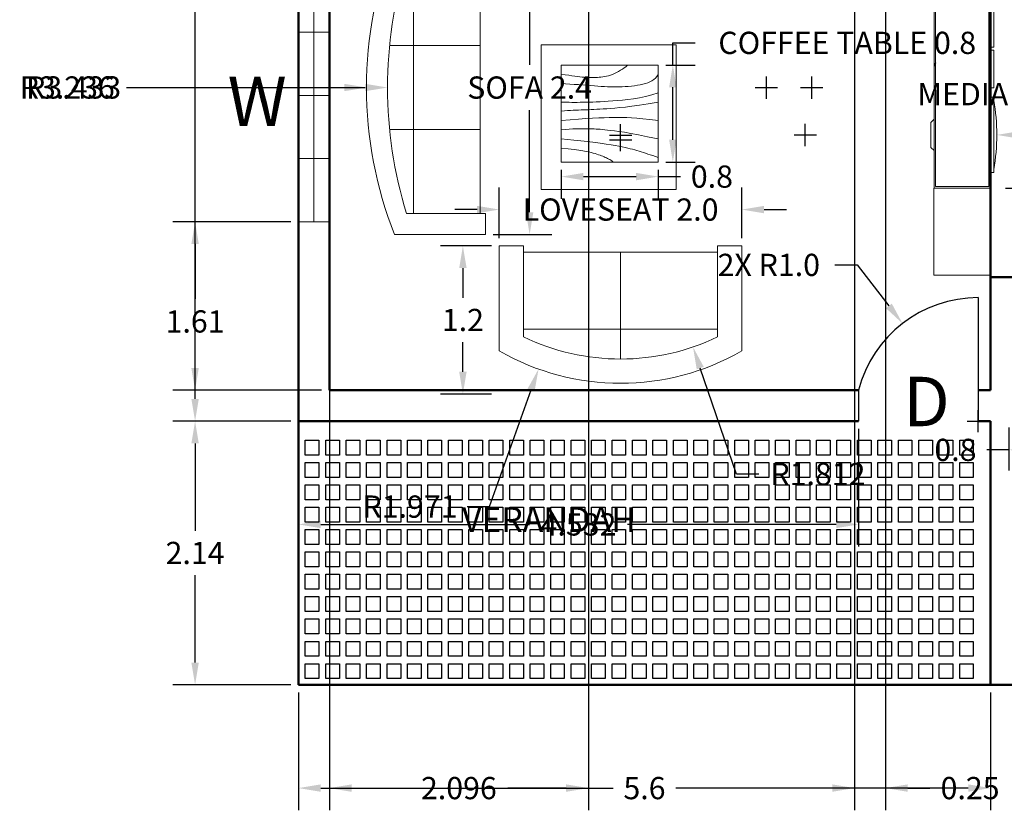
# Model space of a CAD drawing. Units: metres. Extents: x 3.9 to 21.3, y 24.8 to 56.5.
# Tile 1 of 6: x 3.9 to 11.9, y 24.8 to 31.2. Entities that reach past the tile are written whole.
import ezdxf

# ---------------------------------------------------------------- set-up
doc = ezdxf.new("R2010")
doc.units = ezdxf.units.M
doc.header["$MEASUREMENT"] = 0
for name, color, linetype, lineweight in [('A-AREA-IDEN', 3, 'Continuous', 25), ('A-FLOR-PATT', 8, 'Continuous', 13), ('DIMENSIONS', 2, 'Continuous', 18), ('DOOR', 5, 'Continuous', 25), ('FURNITURE', 6, 'Continuous', 18), ('TEXT', 3, 'Continuous', 18), ('WALL', 1, 'Continuous', 50), ('WINDOW', 4, 'Continuous', 18)]:
    doc.layers.add(name, color=color, linetype=linetype, lineweight=lineweight)
doc.styles.get("Standard").update_dxf_attribs({"font": 'arial.ttf'})
doc.dimstyles.get("Standard").update_dxf_attribs({"dimtxt": 0.18, "dimasz": 0.18, "dimexe": 0.18, "dimexo": 0.0625, "dimgap": 0.09, "dimtad": 0, "dimtih": 1, "dimtoh": 1, "dimdec": 1, "dimzin": 0, "dimdsep": 46, "dimtxsty": 'Standard', "dimcen": 0.09, "dimadec": 0, "dimazin": 0, "dimtfac": 1, "dimtdec": 1, "dimtofl": 0, "dimtmove": 0, "dimatfit": 3, "dimfxl": 1, "dimtolj": 1, "dimtzin": 0, "dimarcsym": 0})

# ---------------------------------------------------------------- blocks, each defined once
blk = doc.blocks.new('Entertainment Center')
for p, q in [((-4, 0), (-5, -1)), ((4, 0), (-4, 0)), ((5, -1), (4, 0)), ((-17, -19), (-17, -1)), ((-17, -1), (43, -1)), ((-16.5, -18.5), (-16.5, -1.5)), ((-16.5, -1.5), (42.5, -1.5)), ((42.5, -1.5), (42.5, -18.5)), ((43, -1), (43, -19)), ((42.5, -18.5), (-16.5, -18.5)), ((43, -19), (-17, -19)), ((-12, -20), (-12, -19)), ((12, -20), (-12, -20)), ((12, -19), (12, -20)), ((15, -20), (15, -19)), ((27, -20), (15, -20)), ((27, -19), (27, -20)), ((28, -20), (28, -19)), ((40, -20), (28, -20)), ((40, -19), (40, -20))]:
    blk.add_line(p, q)
blk.add_arc((0, 40), 61, 259.6111, 280.3889)
blk = doc.blocks.new('Sofa - Roundback 7 ft.')
for p, q in [((-12.00002, -32.4421), (-12.00003, -6.5971)), ((11.99997, -32.4421), (11.99998, -6.5971)), ((-36.000027, -34), (-36.000027, -11.4696)), ((-35.999844, -13.3819), (35.9998, -13.3819)), ((35.99998, -34), (35.99998, -11.4696)), ((-36.000027, -32.4421), (35.99998, -32.4421))]:
    blk.add_line(p, q)
for points in [[(-36.000027, -34), (-42.000027, -34), (-42.000027, -8)], [(41.99998, -8), (41.99998, -34), (35.99998, -34)]]:
    blk.add_lwpolyline(points)
for centre, radius, start, end in [((0, -114.25), 114.25, 68.43141, 111.5686), ((-0.00001, -127.1968), 121.1968, 72.72033, 107.2797)]:
    blk.add_arc(centre, radius, start, end)
blk = doc.blocks.new('Sofa - Roundback Loveseat 5 ft.')
for p, q in [((0, -32.44198), (0, -5.99998)), ((-24, -33.99998), (-24, -11.46958)), ((24.00004, -33.99998), (24.00004, -11.46958)), ((-23.9998, -13.38178), (23.99986, -13.38178)), ((-24, -32.44198), (24.00004, -32.44198))]:
    blk.add_line(p, q)
for points in [[(-24, -33.99998), (-30, -33.99998), (-30, -7.99998)], [(30.00004, -7.99998), (30.00004, -33.99998), (24.00004, -33.99998)]]:
    blk.add_lwpolyline(points)
for centre, radius, start, end in [((0, -60.24998), 60.24998, 60.13715, 119.8628), ((0, -61.38438), 55.38444, 64.32083, 115.6792)]:
    blk.add_arc(centre, radius, start, end)
blk = doc.blocks.new('Table - Square Woodgrain 42 x 42 in.')
blk.add_line((0, -42), (42, -42))
for points in [[(0, -4), (1.704, -4.2172), (3.2358, -4.4188), (4.615, -4.604), (5.8615, -4.7721), (6.9951, -4.9224), (8.0357, -5.0541), (9.0031, -5.1667), (9.9171, -5.2594), (10.7951, -5.3316), (11.6445, -5.3836), (12.4702, -5.4157), (13.277, -5.4283), (14.0698, -5.4217), (14.8535, -5.3964), (15.6331, -5.3526), (16.4133, -5.2908), (17.1986, -5.2103), (17.9913, -5.1062), (18.793, -4.9727), (19.6056, -4.8038), (20.4307, -4.5937), (21.2701, -4.3365), (22.1256, -4.0262), (22.9989, -3.6571), (23.888, -3.2272), (24.7756, -2.7516), (25.6408, -2.2491), (26.4624, -1.7387), (27.2195, -1.2395), (27.891, -0.7703), (28.456, -0.3501), (28.8934, 0.002)], [(0, -42), (0, 0), (42, 0), (42, -42)], [(0, -8), (1.8203, -8.1001), (3.6741, -8.2149), (5.5411, -8.3408), (7.4011, -8.4741), (9.2339, -8.6112), (11.0193, -8.7484), (12.7371, -8.8821), (14.3671, -9.0086), (15.8954, -9.1246), (17.3337, -9.2278), (18.6997, -9.3159), (20.0116, -9.387), (21.2871, -9.4389), (22.5442, -9.4696), (23.8008, -9.477), (25.0749, -9.459), (26.3791, -9.4137), (27.7049, -9.3403), (29.0383, -9.2382), (30.3655, -9.1068), (31.6728, -8.9455), (32.9461, -8.7535), (34.1717, -8.5304), (35.3358, -8.2756), (36.4268, -7.9863), (37.443, -7.6521), (38.3849, -7.2603), (39.253, -6.7986), (40.048, -6.2542), (40.7705, -5.6147), (41.421, -4.8674), (42, -4)], [(42, -12), (39.1784, -12.8621), (36.4519, -13.5654), (33.8246, -14.1294), (31.3004, -14.5731), (28.8832, -14.9161), (26.577, -15.1775), (24.3858, -15.3768), (22.3136, -15.5332), (20.3622, -15.6632), (18.5254, -15.7718), (16.7947, -15.8612), (15.1618, -15.9338), (13.6183, -15.9916), (12.1558, -16.0369), (10.7659, -16.0718), (9.4403, -16.0987), (8.1703, -16.1191), (6.9461, -16.1325), (5.7577, -16.1377), (4.595, -16.1335), (3.4479, -16.1188), (2.3064, -16.0924), (1.1604, -16.0532), (0, -16)], [(42, -16), (37.6529, -16.7365), (33.8802, -17.329), (30.6179, -17.7961), (27.8015, -18.1561), (25.3668, -18.4275), (23.2497, -18.6288), (21.3859, -18.7785), (19.7111, -18.8949), (18.1693, -18.9939), (16.7375, -19.0795), (15.401, -19.1534), (14.1449, -19.217), (12.9544, -19.2717), (11.8148, -19.3191), (10.7113, -19.3606), (9.6291, -19.3976), (8.5534, -19.4323), (7.47, -19.4689), (6.3643, -19.5122), (5.222, -19.5672), (4.0288, -19.6386), (2.7703, -19.7313), (1.4321, -19.8501), (0, -20)], [(0, -24), (3.9243, -23.6805), (7.4766, -23.4138), (10.6891, -23.1954), (13.5943, -23.0205), (16.2247, -22.8847), (18.6125, -22.7832), (20.7903, -22.7116), (22.7903, -22.6651), (24.6563, -22.642), (26.4764, -22.6507), (28.35, -22.7024), (30.3766, -22.8084), (32.6555, -22.98), (35.2861, -23.2283), (38.3678, -23.5645), (42, -24)], [(42, -32), (37.392, -31.017), (33.4585, -30.2231), (30.1291, -29.5949), (27.3334, -29.109), (25.0009, -28.742), (23.0612, -28.4707), (21.4439, -28.2716), (20.0786, -28.1215), (18.8998, -28.0002), (17.8609, -27.9014), (16.9206, -27.8219), (16.0371, -27.7588), (15.1691, -27.709), (14.2748, -27.6693), (13.3128, -27.6368), (12.2415, -27.6083), (11.0295, -27.5824), (9.6867, -27.5643), (8.233, -27.5608), (6.6884, -27.5787), (5.0728, -27.6248), (3.4062, -27.7058), (1.7086, -27.8286), (0, -28)], [(0, -32), (5.4026, -32.5358), (9.9494, -33.019), (13.7424, -33.4553), (16.8834, -33.8505), (19.4743, -34.2106), (21.6171, -34.5413), (23.4136, -34.8486), (24.9657, -35.1382), (26.3614, -35.4156), (27.6332, -35.6841), (28.7995, -35.9467), (29.8788, -36.2064), (30.8897, -36.4661), (31.8507, -36.7288), (32.7802, -36.9973), (33.6968, -37.2747), (34.6175, -37.5635), (35.5531, -37.8651), (36.5128, -38.1805), (37.506, -38.5108), (38.5421, -38.8568), (39.6302, -39.2197), (40.7797, -39.6004), (42, -40)], [(0, -36), (3.0098, -36.2857), (5.5354, -36.5643), (7.6368, -36.8359), (9.374, -37.1009), (10.807, -37.3597), (11.9957, -37.6126), (13.0002, -37.8599), (13.8804, -38.102), (14.6874, -38.3393), (15.4365, -38.5729), (16.1338, -38.8041), (16.7858, -39.0341), (17.3987, -39.264), (17.9787, -39.4952), (18.5322, -39.7288), (19.0655, -39.9662), (19.5832, -40.2081), (20.0842, -40.4544), (20.5657, -40.7046), (21.0249, -40.9581), (21.459, -41.2144), (21.8653, -41.4731), (22.2409, -41.7335), (22.5831, -41.9951)]]:
    blk.add_lwpolyline(points)
blk = doc.blocks.new('*U19')
at = {"layer": 'DOOR'}
blk.add_lwpolyline([(-0.0552, 0.0603), (0.0552, 0.0603), (0.0552, -0.0603), (-0.0552, -0.0603)], close=True, dxfattribs=at)
blk = doc.blocks.new('*U20')
at = {"layer": 'A-FLOR-PATT', "transparency": 16777216}
for p in [(0, 1.8102), (0.1655, 1.8102), (0.331, 1.8102), (0.4964, 1.8102), (0.6619, 1.8102), (0.8274, 1.8102), (0.9929, 1.8102), (1.1584, 1.8102), (1.3239, 1.8102), (1.4893, 1.8102), (1.6548, 1.8102), (1.8203, 1.8102), (1.9858, 1.8102), (2.1513, 1.8102), (2.3167, 1.8102), (2.4822, 1.8102), (2.6477, 1.8102), (2.8132, 1.8102), (2.9787, 1.8102), (3.1441, 1.8102), (3.3096, 1.8102), (3.4751, 1.8102), (3.6406, 1.8102), (3.8061, 1.8102), (3.9716, 1.8102), (4.137, 1.8102), (4.3025, 1.8102), (4.468, 1.8102), (4.6335, 1.8102), (4.799, 1.8102), (4.9644, 1.8102), (5.1299, 1.8102), (5.2954, 1.8102), (0, 1.6291), (0.1655, 1.6291), (0.331, 1.6291), (0.4964, 1.6291), (0.6619, 1.6291), (0.8274, 1.6291), (0.9929, 1.6291), (1.1584, 1.6291), (1.3239, 1.6291), (1.4893, 1.6291), (1.6548, 1.6291), (1.8203, 1.6291), (1.9858, 1.6291), (2.1513, 1.6291), (2.3167, 1.6291), (2.4822, 1.6291), (2.6477, 1.6291), (2.8132, 1.6291), (2.9787, 1.6291), (3.1441, 1.6291), (3.3096, 1.6291), (3.4751, 1.6291), (3.6406, 1.6291), (3.8061, 1.6291), (3.9716, 1.6291), (4.137, 1.6291), (4.3025, 1.6291), (4.468, 1.6291), (4.6335, 1.6291), (4.799, 1.6291), (4.9644, 1.6291), (5.1299, 1.6291), (5.2954, 1.6291), (0, 1.4481), (0.1655, 1.4481), (0.331, 1.4481), (0.4964, 1.4481), (0.6619, 1.4481), (0.8274, 1.4481), (0.9929, 1.4481), (1.1584, 1.4481), (1.3239, 1.4481), (1.4893, 1.4481), (1.6548, 1.4481), (1.8203, 1.4481), (1.9858, 1.4481), (2.1513, 1.4481), (2.3167, 1.4481), (2.4822, 1.4481), (2.6477, 1.4481), (2.8132, 1.4481), (2.9787, 1.4481), (3.1441, 1.4481), (3.3096, 1.4481), (3.4751, 1.4481), (3.6406, 1.4481), (3.8061, 1.4481), (3.9716, 1.4481), (4.137, 1.4481), (4.3025, 1.4481), (4.468, 1.4481), (4.6335, 1.4481), (4.799, 1.4481), (4.9644, 1.4481), (5.1299, 1.4481), (5.2954, 1.4481), (0, 1.2671), (0.1655, 1.2671), (0.331, 1.2671), (0.4964, 1.2671), (0.6619, 1.2671), (0.8274, 1.2671), (0.9929, 1.2671), (1.1584, 1.2671), (1.3239, 1.2671), (1.4893, 1.2671), (1.6548, 1.2671), (1.8203, 1.2671), (1.9858, 1.2671), (2.1513, 1.2671), (2.3167, 1.2671), (2.4822, 1.2671), (2.6477, 1.2671), (2.8132, 1.2671), (2.9787, 1.2671), (3.1441, 1.2671), (3.3096, 1.2671), (3.4751, 1.2671), (3.6406, 1.2671), (3.8061, 1.2671), (3.9716, 1.2671), (4.137, 1.2671), (4.3025, 1.2671), (4.468, 1.2671), (4.6335, 1.2671), (4.799, 1.2671), (4.9644, 1.2671), (5.1299, 1.2671), (5.2954, 1.2671), (0, 1.0861), (0.1655, 1.0861), (0.331, 1.0861), (0.4964, 1.0861), (0.6619, 1.0861), (0.8274, 1.0861), (0.9929, 1.0861), (1.1584, 1.0861), (1.3239, 1.0861), (1.4893, 1.0861), (1.6548, 1.0861), (1.8203, 1.0861), (1.9858, 1.0861), (2.1513, 1.0861), (2.3167, 1.0861), (2.4822, 1.0861), (2.6477, 1.0861), (2.8132, 1.0861), (2.9787, 1.0861), (3.1441, 1.0861), (3.3096, 1.0861), (3.4751, 1.0861), (3.6406, 1.0861), (3.8061, 1.0861), (3.9716, 1.0861), (4.137, 1.0861), (4.3025, 1.0861), (4.468, 1.0861), (4.6335, 1.0861), (4.799, 1.0861), (4.9644, 1.0861), (5.1299, 1.0861), (5.2954, 1.0861), (0, 0.9051), (0.1655, 0.9051), (0.331, 0.9051), (0.4964, 0.9051), (0.6619, 0.9051), (0.8274, 0.9051), (0.9929, 0.9051), (1.1584, 0.9051), (1.3239, 0.9051), (1.4893, 0.9051), (1.6548, 0.9051), (1.8203, 0.9051), (1.9858, 0.9051), (2.1513, 0.9051), (2.3167, 0.9051), (2.4822, 0.9051), (2.6477, 0.9051), (2.8132, 0.9051), (2.9787, 0.9051), (3.1441, 0.9051), (3.3096, 0.9051), (3.4751, 0.9051), (3.6406, 0.9051), (3.8061, 0.9051), (3.9716, 0.9051), (4.137, 0.9051), (4.3025, 0.9051), (4.468, 0.9051), (4.6335, 0.9051), (4.799, 0.9051), (4.9644, 0.9051), (5.1299, 0.9051), (5.2954, 0.9051), (0, 0.7241), (0.1655, 0.7241), (0.331, 0.7241), (0.4964, 0.7241), (0.6619, 0.7241), (0.8274, 0.7241), (0.9929, 0.7241), (1.1584, 0.7241), (1.3239, 0.7241), (1.4893, 0.7241), (1.6548, 0.7241), (1.8203, 0.7241), (1.9858, 0.7241), (2.1513, 0.7241), (2.3167, 0.7241), (2.4822, 0.7241), (2.6477, 0.7241), (2.8132, 0.7241), (2.9787, 0.7241), (3.1441, 0.7241), (3.3096, 0.7241), (3.4751, 0.7241), (3.6406, 0.7241), (3.8061, 0.7241), (3.9716, 0.7241), (4.137, 0.7241), (4.3025, 0.7241), (4.468, 0.7241), (4.6335, 0.7241), (4.799, 0.7241), (4.9644, 0.7241), (5.1299, 0.7241), (5.2954, 0.7241), (0, 0.543), (0.1655, 0.543), (0.331, 0.543), (0.4964, 0.543), (0.6619, 0.543), (0.8274, 0.543), (0.9929, 0.543), (1.1584, 0.543), (1.3239, 0.543), (1.4893, 0.543), (1.6548, 0.543), (1.8203, 0.543), (1.9858, 0.543), (2.1513, 0.543), (2.3167, 0.543), (2.4822, 0.543), (2.6477, 0.543), (2.8132, 0.543), (2.9787, 0.543), (3.1441, 0.543), (3.3096, 0.543), (3.4751, 0.543), (3.6406, 0.543), (3.8061, 0.543), (3.9716, 0.543), (4.137, 0.543), (4.3025, 0.543), (4.468, 0.543), (4.6335, 0.543), (4.799, 0.543), (4.9644, 0.543), (5.1299, 0.543), (5.2954, 0.543), (0, 0.362), (0.1655, 0.362), (0.331, 0.362), (0.4964, 0.362), (0.6619, 0.362), (0.8274, 0.362), (0.9929, 0.362), (1.1584, 0.362), (1.3239, 0.362), (1.4893, 0.362), (1.6548, 0.362), (1.8203, 0.362), (1.9858, 0.362), (2.1513, 0.362), (2.3167, 0.362), (2.4822, 0.362), (2.6477, 0.362), (2.8132, 0.362), (2.9787, 0.362), (3.1441, 0.362), (3.3096, 0.362), (3.4751, 0.362), (3.6406, 0.362), (3.8061, 0.362), (3.9716, 0.362), (4.137, 0.362), (4.3025, 0.362), (4.468, 0.362), (4.6335, 0.362), (4.799, 0.362), (4.9644, 0.362), (5.1299, 0.362), (5.2954, 0.362), (0, 0.181), (0.1655, 0.181), (0.331, 0.181), (0.4964, 0.181), (0.6619, 0.181), (0.8274, 0.181), (0.9929, 0.181), (1.1584, 0.181), (1.3239, 0.181), (1.4893, 0.181), (1.6548, 0.181), (1.8203, 0.181), (1.9858, 0.181), (2.1513, 0.181), (2.3167, 0.181), (2.4822, 0.181), (2.6477, 0.181), (2.8132, 0.181), (2.9787, 0.181), (3.1441, 0.181), (3.3096, 0.181), (3.4751, 0.181), (3.6406, 0.181), (3.8061, 0.181), (3.9716, 0.181), (4.137, 0.181), (4.3025, 0.181), (4.468, 0.181), (4.6335, 0.181), (4.799, 0.181), (4.9644, 0.181), (5.1299, 0.181), (5.2954, 0.181), (0, 0), (0.1655, 0), (0.331, 0), (0.4964, 0), (0.6619, 0), (0.8274, 0), (0.9929, 0), (1.1584, 0), (1.3239, 0), (1.4893, 0), (1.6548, 0), (1.8203, 0), (1.9858, 0), (2.1513, 0), (2.3167, 0), (2.4822, 0), (2.6477, 0), (2.8132, 0), (2.9787, 0), (3.1441, 0), (3.3096, 0), (3.4751, 0), (3.6406, 0), (3.8061, 0), (3.9716, 0), (4.137, 0), (4.3025, 0), (4.468, 0), (4.6335, 0), (4.799, 0), (4.9644, 0), (5.1299, 0), (5.2954, 0)]:
    blk.add_blockref('*U19', p, dxfattribs=at)
blk = doc.blocks.new('WIN-4-LIGHT-2046')
for p, q in [((0.5115, -0.125), (0, -0.125)), ((0.5115, -0.125), (1.0231, -0.125)), ((1.5346, -0.125), (1.0231, -0.125)), ((1.5346, -0.125), (2.0462, -0.125))]:
    blk.add_line(p, q)
for points in [[(0.5115, 0), (0, 0), (0, -0.25), (0.5115, -0.25)], [(0.5115, 0), (1.0231, 0), (1.0231, -0.25), (0.5115, -0.25)], [(1.5346, 0), (1.0231, 0), (1.0231, -0.25), (1.5346, -0.25)], [(1.5346, 0), (2.0462, 0), (2.0462, -0.25), (1.5346, -0.25)]]:
    blk.add_lwpolyline(points, close=True)
blk = doc.blocks.new('*D59')
at = {"layer": 'Defpoints', "color": 0, "transparency": 16777216}
for p in [(11.8164, 31.3903), (12.045, 31.3903), (11.8164, 29.8663)]:
    blk.add_point(p, dxfattribs=at)
at = {"layer": 'DIMENSIONS', "color": 0, "lineweight": -2, "transparency": 16777216}
for p, q in [((11.8789, 31.3903), (12.225, 31.3903)), ((12.045, 31.2103), (12.045, 30.8102)), ((12.045, 30.0463), (12.045, 30.4464)), ((11.8789, 29.8663), (12.225, 29.8663))]:
    blk.add_line(p, q, dxfattribs=at)
at = {"layer": 'DIMENSIONS', "color": 0, "transparency": 16777216}
for points in [[(12.015, 31.2103), (12.075, 31.2103), (12.045, 31.3903)], [(12.015, 30.0463), (12.075, 30.0463), (12.045, 29.8663)]]:
    blk.add_solid(points, dxfattribs=at)
at = {"layer": 'DIMENSIONS', "color": 0, "transparency": 16777216, "insert": (12.045, 30.6283), "char_height": 0.18, "attachment_point": 5}
blk.add_mtext('\\A1;MEDIA UNIT 1.5', dxfattribs=at)
blk = doc.blocks.new('*D61')
at = {"layer": 'Defpoints', "color": 0, "transparency": 16777216}
for p in [(7.6708, 31.8712), (8.0277, 31.8712), (7.6708, 29.4918)]:
    blk.add_point(p, dxfattribs=at)
at = {"layer": 'DIMENSIONS', "color": 0, "lineweight": -2, "transparency": 16777216}
for p, q in [((7.7333, 31.8712), (8.2077, 31.8712)), ((8.0277, 31.6912), (8.0277, 30.8646)), ((8.0277, 29.6718), (8.0277, 30.4984)), ((7.7333, 29.4918), (8.2077, 29.4918))]:
    blk.add_line(p, q, dxfattribs=at)
at = {"layer": 'DIMENSIONS', "color": 0, "transparency": 16777216}
for points in [[(7.9977, 31.6912), (8.0577, 31.6912), (8.0277, 31.8712)], [(7.9977, 29.6718), (8.0577, 29.6718), (8.0277, 29.4918)]]:
    blk.add_solid(points, dxfattribs=at)
at = {"layer": 'DIMENSIONS', "color": 0, "transparency": 16777216, "insert": (8.0277, 30.6815), "char_height": 0.18, "attachment_point": 5}
blk.add_mtext('\\A1;SOFA 2.4', dxfattribs=at)
blk = doc.blocks.new('*D63')
at = {"layer": 'Defpoints', "color": 0, "transparency": 16777216}
for p in [(7.7822, 29.6935), (7.7822, 29.399), (9.7451, 29.399)]:
    blk.add_point(p, dxfattribs=at)
at = {"layer": 'DIMENSIONS', "color": 0, "lineweight": -2, "transparency": 16777216}
for p, q in [((7.7822, 29.4615), (7.7822, 29.8735)), ((9.7451, 29.4615), (9.7451, 29.8735)), ((7.6022, 29.6935), (7.4222, 29.6935)), ((9.9251, 29.6935), (10.1051, 29.6935))]:
    blk.add_line(p, q, dxfattribs=at)
at = {"layer": 'DIMENSIONS', "color": 0, "transparency": 16777216}
for points in [[(7.6022, 29.7235), (7.6022, 29.6635), (7.7822, 29.6935)], [(9.9251, 29.7235), (9.9251, 29.6635), (9.7451, 29.6935)]]:
    blk.add_solid(points, dxfattribs=at)
at = {"layer": 'DIMENSIONS', "color": 0, "transparency": 16777216, "insert": (8.7636, 29.6935), "char_height": 0.18, "attachment_point": 5}
blk.add_mtext('\\A1;LOVESEAT 2.0', dxfattribs=at)
blk = doc.blocks.new('*D64')
at = {"layer": 'Defpoints', "color": 0, "transparency": 16777216}
for p in [(7.7822, 29.399), (7.4878, 28.1995), (7.7822, 28.1995)]:
    blk.add_point(p, dxfattribs=at)
at = {"layer": 'DIMENSIONS', "color": 0, "lineweight": -2, "transparency": 16777216}
for p, q in [((7.7197, 29.399), (7.3078, 29.399)), ((7.4878, 29.219), (7.4878, 28.9797)), ((7.4878, 28.3795), (7.4878, 28.6189)), ((7.7197, 28.1995), (7.3078, 28.1995))]:
    blk.add_line(p, q, dxfattribs=at)
at = {"layer": 'DIMENSIONS', "color": 0, "transparency": 16777216}
for points in [[(7.4578, 29.219), (7.5178, 29.219), (7.4878, 29.399)], [(7.4578, 28.3795), (7.5178, 28.3795), (7.4878, 28.1995)]]:
    blk.add_solid(points, dxfattribs=at)
at = {"layer": 'DIMENSIONS', "color": 0, "transparency": 16777216, "insert": (7.4878, 28.7993), "char_height": 0.18, "attachment_point": 5}
blk.add_mtext('\\A1;1.2', dxfattribs=at)
blk = doc.blocks.new('*D65')
at = {"layer": 'Defpoints', "color": 0, "transparency": 16777216}
for p in [(9.0686, 30.8635), (9.1864, 30.8635), (9.0686, 30.0783)]:
    blk.add_point(p, dxfattribs=at)
at = {"layer": 'DIMENSIONS', "color": 0, "lineweight": -2, "transparency": 16777216}
for p, q in [((9.1864, 30.8635), (9.1864, 31.0435)), ((9.1864, 31.0435), (9.3664, 31.0435)), ((9.1311, 30.8635), (9.3664, 30.8635)), ((9.1864, 30.2583), (9.1864, 30.6835)), ((9.1311, 30.0783), (9.3664, 30.0783))]:
    blk.add_line(p, q, dxfattribs=at)
at = {"layer": 'DIMENSIONS', "color": 0, "transparency": 16777216}
for points in [[(9.1564, 30.6835), (9.2164, 30.6835), (9.1864, 30.8635)], [(9.1564, 30.2583), (9.2164, 30.2583), (9.1864, 30.0783)]]:
    blk.add_solid(points, dxfattribs=at)
at = {"layer": 'DIMENSIONS', "color": 0, "transparency": 16777216, "insert": (10.5975, 31.0435), "char_height": 0.18, "attachment_point": 5}
blk.add_mtext('\\A1;COFFEE TABLE 0.8', dxfattribs=at)
blk = doc.blocks.new('*D66')
at = {"layer": 'Defpoints', "color": 0, "transparency": 16777216}
for p in [(8.2835, 30.0783), (9.0686, 30.0783), (9.0686, 29.9605)]:
    blk.add_point(p, dxfattribs=at)
at = {"layer": 'DIMENSIONS', "color": 0, "lineweight": -2, "transparency": 16777216}
for p, q in [((8.2835, 30.0158), (8.2835, 29.7805)), ((8.4635, 29.9605), (8.8886, 29.9605)), ((9.0686, 30.0158), (9.0686, 29.7805)), ((9.0686, 29.9605), (9.2486, 29.9605))]:
    blk.add_line(p, q, dxfattribs=at)
at = {"layer": 'DIMENSIONS', "color": 0, "transparency": 16777216}
for points in [[(8.4635, 29.9905), (8.4635, 29.9305), (8.2835, 29.9605)], [(8.8886, 29.9905), (8.8886, 29.9305), (9.0686, 29.9605)]]:
    blk.add_solid(points, dxfattribs=at)
at = {"layer": 'DIMENSIONS', "color": 0, "transparency": 16777216, "insert": (9.5027, 29.9605), "char_height": 0.18, "attachment_point": 5}
blk.add_mtext('\\A1;0.8', dxfattribs=at)
blk = doc.blocks.new('*D72')
at = {"layer": 'Defpoints', "color": 0, "transparency": 16777216}
for p in [(11.9074, 27.7476), (11.9074, 27.519), (12.6694, 27.519)]:
    blk.add_point(p, dxfattribs=at)
at = {"layer": 'DIMENSIONS', "color": 0, "lineweight": -2, "transparency": 16777216}
for p, q in [((11.9074, 27.5815), (11.9074, 27.9276)), ((12.6694, 27.5815), (12.6694, 27.9276)), ((11.9074, 27.7476), (11.7274, 27.7476)), ((12.4894, 27.7476), (12.0874, 27.7476))]:
    blk.add_line(p, q, dxfattribs=at)
at = {"layer": 'DIMENSIONS', "color": 0, "transparency": 16777216}
for points in [[(12.0874, 27.7776), (12.0874, 27.7176), (11.9074, 27.7476)], [(12.4894, 27.7776), (12.4894, 27.7176), (12.6694, 27.7476)]]:
    blk.add_solid(points, dxfattribs=at)
at = {"layer": 'DIMENSIONS', "color": 0, "transparency": 16777216, "insert": (11.4733, 27.7476), "char_height": 0.18, "attachment_point": 5}
blk.add_mtext('\\A1;0.8', dxfattribs=at)
blk = doc.blocks.new('*D73')
at = {"layer": 'Defpoints', "color": 0, "transparency": 16777216}
for p in [(5.3206, 27.9803), (6.1571, 27.9803), (6.1571, 25.8451)]:
    blk.add_point(p, dxfattribs=at)
at = {"layer": 'DIMENSIONS', "color": 0, "lineweight": -2, "transparency": 16777216}
for p, q in [((6.0946, 27.9803), (5.1406, 27.9803)), ((5.3206, 27.8003), (5.3206, 27.0931)), ((5.3206, 26.0251), (5.3206, 26.7323)), ((6.0946, 25.8451), (5.1406, 25.8451))]:
    blk.add_line(p, q, dxfattribs=at)
at = {"layer": 'DIMENSIONS', "color": 0, "transparency": 16777216}
for points in [[(5.2906, 27.8003), (5.3506, 27.8003), (5.3206, 27.9803)], [(5.2906, 26.0251), (5.3506, 26.0251), (5.3206, 25.8451)]]:
    blk.add_solid(points, dxfattribs=at)
at = {"layer": 'DIMENSIONS', "color": 0, "transparency": 16777216, "insert": (5.3206, 26.9127), "char_height": 0.18, "attachment_point": 5}
blk.add_mtext('\\A1;2.14', dxfattribs=at)
blk = doc.blocks.new('*D74')
at = {"layer": 'Defpoints', "color": 0, "transparency": 16777216}
for p in [(6.1571, 25.8451), (11.7571, 25.8451), (11.7571, 25.0086)]:
    blk.add_point(p, dxfattribs=at)
at = {"layer": 'DIMENSIONS', "color": 0, "lineweight": -2, "transparency": 16777216}
for p, q in [((6.1571, 25.7826), (6.1571, 24.8286)), ((11.7571, 25.7826), (11.7571, 24.8286)), ((6.3371, 25.0086), (8.7033, 25.0086)), ((11.5771, 25.0086), (9.2109, 25.0086))]:
    blk.add_line(p, q, dxfattribs=at)
at = {"layer": 'DIMENSIONS', "color": 0, "transparency": 16777216}
for points in [[(6.3371, 25.0386), (6.3371, 24.9786), (6.1571, 25.0086)], [(11.5771, 25.0386), (11.5771, 24.9786), (11.7571, 25.0086)]]:
    blk.add_solid(points, dxfattribs=at)
at = {"layer": 'DIMENSIONS', "color": 0, "transparency": 16777216, "insert": (8.9571, 25.0086), "char_height": 0.18, "attachment_point": 5}
blk.add_mtext('\\A1;5.6', dxfattribs=at)
blk = doc.blocks.new('*D76')
at = {"layer": 'Defpoints', "color": 0, "transparency": 16777216}
for p in [(6.4071, 38.6451), (5.3206, 28.2303), (6.4071, 28.2303)]:
    blk.add_point(p, dxfattribs=at)
at = {"layer": 'DIMENSIONS', "color": 0, "lineweight": -2, "transparency": 16777216}
for p, q in [((6.3446, 38.6451), (5.1406, 38.6451)), ((5.3206, 38.4651), (5.3206, 33.6196)), ((5.3206, 28.4103), (5.3206, 33.2558)), ((6.3446, 28.2303), (5.1406, 28.2303))]:
    blk.add_line(p, q, dxfattribs=at)
at = {"layer": 'DIMENSIONS', "color": 0, "transparency": 16777216}
for points in [[(5.2906, 38.4651), (5.3506, 38.4651), (5.3206, 38.6451)], [(5.2906, 28.4103), (5.3506, 28.4103), (5.3206, 28.2303)]]:
    blk.add_solid(points, dxfattribs=at)
at = {"layer": 'DIMENSIONS', "color": 0, "transparency": 16777216, "insert": (5.3206, 33.4377), "char_height": 0.18, "attachment_point": 5}
blk.add_mtext('\\A1;10.415', dxfattribs=at)
blk = doc.blocks.new('*D79')
at = {"layer": 'Defpoints', "color": 0, "transparency": 16777216}
for p in [(10.6571, 32.2457), (10.9071, 32.2457), (10.9071, 25.0086)]:
    blk.add_point(p, dxfattribs=at)
at = {"layer": 'DIMENSIONS', "color": 0, "lineweight": -2, "transparency": 16777216}
for p, q in [((10.6571, 32.1832), (10.6571, 24.8286)), ((10.9071, 32.1832), (10.9071, 24.8286)), ((10.4771, 25.0086), (10.2971, 25.0086)), ((11.0871, 25.0086), (11.2671, 25.0086))]:
    blk.add_line(p, q, dxfattribs=at)
at = {"layer": 'DIMENSIONS', "color": 0, "transparency": 16777216}
for points in [[(10.4771, 25.0386), (10.4771, 24.9786), (10.6571, 25.0086)], [(11.0871, 25.0386), (11.0871, 24.9786), (10.9071, 25.0086)]]:
    blk.add_solid(points, dxfattribs=at)
at = {"layer": 'DIMENSIONS', "color": 0, "transparency": 16777216, "insert": (11.5916, 25.0086), "char_height": 0.18, "attachment_point": 5}
blk.add_mtext('\\A1;0.25', dxfattribs=at)
blk = doc.blocks.new('*D91')
at = {"layer": 'Defpoints', "color": 0, "transparency": 16777216}
for p in [(5.3206, 29.5947), (6.1571, 29.5947), (6.1571, 27.9803)]:
    blk.add_point(p, dxfattribs=at)
at = {"layer": 'DIMENSIONS', "color": 0, "lineweight": -2, "transparency": 16777216}
for p, q in [((6.0946, 29.5947), (5.1406, 29.5947)), ((5.3206, 29.4147), (5.3206, 28.9694)), ((5.3206, 28.1603), (5.3206, 28.6056)), ((6.0946, 27.9803), (5.1406, 27.9803))]:
    blk.add_line(p, q, dxfattribs=at)
at = {"layer": 'DIMENSIONS', "color": 0, "transparency": 16777216}
for points in [[(5.2906, 29.4147), (5.3506, 29.4147), (5.3206, 29.5947)], [(5.2906, 28.1603), (5.3506, 28.1603), (5.3206, 27.9803)]]:
    blk.add_solid(points, dxfattribs=at)
at = {"layer": 'DIMENSIONS', "color": 0, "transparency": 16777216, "insert": (5.3206, 28.7875), "char_height": 0.18, "attachment_point": 5}
blk.add_mtext('\\A1;1.61', dxfattribs=at)
blk = doc.blocks.new('*D96')
at = {"layer": 'Defpoints', "color": 0, "transparency": 16777216}
for p in [(6.4071, 35.5686), (8.5033, 35.5686), (8.5033, 25.0086)]:
    blk.add_point(p, dxfattribs=at)
at = {"layer": 'DIMENSIONS', "color": 0, "lineweight": -2, "transparency": 16777216}
for p, q in [((6.4071, 35.5061), (6.4071, 24.8286)), ((8.5033, 35.5061), (8.5033, 24.8286)), ((6.5871, 25.0086), (7.06, 25.0086)), ((8.3233, 25.0086), (7.8504, 25.0086))]:
    blk.add_line(p, q, dxfattribs=at)
at = {"layer": 'DIMENSIONS', "color": 0, "transparency": 16777216}
for points in [[(6.5871, 25.0386), (6.5871, 24.9786), (6.4071, 25.0086)], [(8.3233, 25.0386), (8.3233, 24.9786), (8.5033, 25.0086)]]:
    blk.add_solid(points, dxfattribs=at)
at = {"layer": 'DIMENSIONS', "color": 0, "transparency": 16777216, "insert": (7.4552, 25.0086), "char_height": 0.18, "attachment_point": 5}
blk.add_mtext('\\A1;2.096', dxfattribs=at)
blk = doc.blocks.new('*D101')
at = {"layer": 'Defpoints', "color": 0, "transparency": 16777216}
for p in [(6.1571, 27.9803), (10.6889, 27.9803), (6.1571, 27.1438)]:
    blk.add_point(p, dxfattribs=at)
at = {"layer": 'DIMENSIONS', "color": 0, "lineweight": -2, "transparency": 16777216}
for p, q in [((6.1571, 27.9178), (6.1571, 26.9638)), ((10.6889, 27.9178), (10.6889, 26.9638)), ((6.3371, 27.1438), (8.0266, 27.1438)), ((10.5089, 27.1438), (8.8194, 27.1438))]:
    blk.add_line(p, q, dxfattribs=at)
at = {"layer": 'DIMENSIONS', "color": 0, "transparency": 16777216}
for points in [[(6.3371, 27.1738), (6.3371, 27.1138), (6.1571, 27.1438)], [(10.5089, 27.1738), (10.5089, 27.1138), (10.6889, 27.1438)]]:
    blk.add_solid(points, dxfattribs=at)
at = {"layer": 'DIMENSIONS', "color": 0, "transparency": 16777216, "insert": (8.423, 27.1438), "char_height": 0.18, "attachment_point": 5}
blk.add_mtext('\\A1;4.532', dxfattribs=at)
blk = doc.blocks.new('*D103')
at = {"layer": 'Defpoints', "color": 0, "transparency": 16777216}
for p in [(11.045, 28.771), (11.6571, 27.9803)]:
    blk.add_point(p, dxfattribs=at)
at = {"layer": 'DIMENSIONS', "color": 0, "lineweight": -2, "transparency": 16777216}
for p, q in [((10.4977, 29.2455), (10.6777, 29.2455)), ((10.6777, 29.2455), (10.9348, 28.9134)), ((11.6571, 27.8903), (11.6571, 28.0703)), ((11.5671, 27.9803), (11.7471, 27.9803))]:
    blk.add_line(p, q, dxfattribs=at)
at = {"layer": 'DIMENSIONS', "color": 0, "transparency": 16777216}
blk.add_solid([(10.9585, 28.9317), (10.9111, 28.895), (11.045, 28.771)], dxfattribs=at)
at = {"layer": 'DIMENSIONS', "color": 0, "transparency": 16777216, "insert": (9.9631, 29.2455), "char_height": 0.18, "attachment_point": 5}
blk.add_mtext('\\A1;2X R1.0', dxfattribs=at)
blk = doc.blocks.new('*D107')
at = {"layer": 'Defpoints', "color": 0, "transparency": 16777216}
for p in [(6.8776, 30.682), (10.3106, 30.6815)]:
    blk.add_point(p, dxfattribs=at)
at = {"layer": 'DIMENSIONS', "color": 0, "lineweight": -2, "transparency": 16777216}
for p, q in [((10.3106, 30.5915), (10.3106, 30.7715)), ((4.8178, 30.6823), (6.6976, 30.682)), ((10.2206, 30.6815), (10.4006, 30.6815))]:
    blk.add_line(p, q, dxfattribs=at)
at = {"layer": 'DIMENSIONS', "color": 0, "transparency": 16777216}
blk.add_solid([(6.6976, 30.712), (6.6976, 30.652), (6.8776, 30.682)], dxfattribs=at)
at = {"layer": 'DIMENSIONS', "color": 0, "transparency": 16777216, "insert": (4.338, 30.6823), "char_height": 0.18, "attachment_point": 5}
blk.add_mtext('\\A1;R3.433', dxfattribs=at)
blk = doc.blocks.new('*D108')
at = {"layer": 'Defpoints', "color": 0, "transparency": 16777216}
for p in [(6.7077, 30.682), (9.9439, 30.6815)]:
    blk.add_point(p, dxfattribs=at)
at = {"layer": 'DIMENSIONS', "color": 0, "lineweight": -2, "transparency": 16777216}
for p, q in [((9.9439, 30.5915), (9.9439, 30.7715)), ((4.7659, 30.6823), (6.5277, 30.682)), ((9.8539, 30.6815), (10.0339, 30.6815))]:
    blk.add_line(p, q, dxfattribs=at)
at = {"layer": 'DIMENSIONS', "color": 0, "transparency": 16777216}
blk.add_solid([(6.5277, 30.712), (6.5277, 30.652), (6.7077, 30.682)], dxfattribs=at)
at = {"layer": 'DIMENSIONS', "color": 0, "transparency": 16777216, "insert": (4.2862, 30.6823), "char_height": 0.18, "attachment_point": 5}
blk.add_mtext('\\A1;R3.236', dxfattribs=at)
blk = doc.blocks.new('*D109')
at = {"layer": 'Defpoints', "color": 0, "transparency": 16777216}
for p in [(8.7636, 30.2578), (8.1, 28.4019)]:
    blk.add_point(p, dxfattribs=at)
at = {"layer": 'DIMENSIONS', "color": 0, "lineweight": -2, "transparency": 16777216}
for p, q in [((8.7636, 30.1678), (8.7636, 30.3478)), ((8.6736, 30.2578), (8.8536, 30.2578)), ((7.7017, 27.2883), (8.0393, 28.2324)), ((7.5217, 27.2883), (7.7017, 27.2883))]:
    blk.add_line(p, q, dxfattribs=at)
at = {"layer": 'DIMENSIONS', "color": 0, "transparency": 16777216}
blk.add_solid([(8.0111, 28.2425), (8.0676, 28.2223), (8.1, 28.4019)], dxfattribs=at)
at = {"layer": 'DIMENSIONS', "color": 0, "transparency": 16777216, "insert": (7.0593, 27.2883), "char_height": 0.18, "attachment_point": 5}
blk.add_mtext('\\A1;R1.971', dxfattribs=at)
blk = doc.blocks.new('*D110')
at = {"layer": 'Defpoints', "color": 0, "transparency": 16777216}
for p in [(8.7636, 30.2949), (9.3498, 28.5805)]:
    blk.add_point(p, dxfattribs=at)
at = {"layer": 'DIMENSIONS', "color": 0, "lineweight": -2, "transparency": 16777216}
for p, q in [((8.7636, 30.2049), (8.7636, 30.3849)), ((8.6736, 30.2949), (8.8536, 30.2949)), ((9.7015, 27.5519), (9.4081, 28.4102)), ((9.8815, 27.5519), (9.7015, 27.5519))]:
    blk.add_line(p, q, dxfattribs=at)
at = {"layer": 'DIMENSIONS', "color": 0, "transparency": 16777216}
blk.add_solid([(9.4365, 28.4199), (9.3797, 28.4005), (9.3498, 28.5805)], dxfattribs=at)
at = {"layer": 'DIMENSIONS', "color": 0, "transparency": 16777216, "insert": (10.3605, 27.5519), "char_height": 0.18, "attachment_point": 5}
blk.add_mtext('\\A1;R1.812', dxfattribs=at)
blk = doc.blocks.new('*D111')
at = {"layer": 'Defpoints', "color": 0, "transparency": 16777216}
for p in [(10.2586, 30.2981), (11.808, 30.298)]:
    blk.add_point(p, dxfattribs=at)
at = {"layer": 'DIMENSIONS', "color": 0, "lineweight": -2, "transparency": 16777216}
for p, q in [((10.2586, 30.2081), (10.2586, 30.3881)), ((10.1686, 30.2981), (10.3486, 30.2981)), ((12.7376, 30.2979), (11.988, 30.298))]:
    blk.add_line(p, q, dxfattribs=at)
at = {"layer": 'DIMENSIONS', "color": 0, "transparency": 16777216}
blk.add_solid([(11.988, 30.328), (11.988, 30.268), (11.808, 30.298)], dxfattribs=at)
at = {"layer": 'DIMENSIONS', "color": 0, "transparency": 16777216, "insert": (13.1482, 30.2979), "char_height": 0.18, "attachment_point": 5}
blk.add_mtext('\\A1;R1.55', dxfattribs=at)

msp = doc.modelspace()

# ---------------------------------------------------------------- linework, layer by layer
at = {"layer": 'DOOR'}
for p, q in [((11.6571, 28.9803), (11.6571, 27.9803)), ((10.6889, 28.2303), (10.6889, 27.9803))]:
    msp.add_line(p, q, dxfattribs=at)
for centre, radius, start, end in [((12.1168, 30.4682), 0.904, 152.82202, 154.64088), ((11.6571, 27.9803), 1, 90, 165.52249)]:
    msp.add_arc(centre, radius, start, end, dxfattribs=at)
at = {"layer": 'FURNITURE'}
for points in [[(8.1215, 31.0287), (9.2141, 31.0287), (9.2141, 29.8547), (8.1215, 29.8547)], [(11.7572, 29.8663), (11.2972, 29.8663), (11.2972, 29.1628), (11.7572, 29.1628)]]:
    msp.add_lwpolyline(points, close=True, dxfattribs=at)
at = {"layer": 'WALL'}
for p, q in [((6.1571, 25.8451), (6.1571, 38.8951)), ((6.4071, 28.2303), (6.4071, 38.6451)), ((11.7571, 28.2303), (11.7571, 32.1457)), ((11.7571, 29.1451), (12.0071, 29.1451)), ((6.4071, 28.2303), (10.6889, 28.2303)), ((11.6571, 28.2303), (11.7571, 28.2303)), ((6.1571, 27.9803), (10.6889, 27.9803)), ((11.6571, 27.9803), (11.7571, 27.9803)), ((11.7571, 25.8451), (11.7571, 27.9803)), ((6.1571, 25.8451), (15.7571, 25.8451))]:
    msp.add_line(p, q, dxfattribs=at)

# ---------------------------------------------------------------- block references
at = {"layer": 'A-FLOR-PATT'}
msp.add_blockref('*U20', (6.2674, 25.9557), dxfattribs=at)
at = {"layer": 'FURNITURE'}
for name, p, xscale, yscale, zscale, rotation in [('Sofa - Roundback 7 ft.', (6.7077, 30.6815), 0.0283257265101147, 0.0283257265101147, 0.0283257265101147, 89.99997936313675), ('Entertainment Center', (11.2746, 30.2981), 0.0254, 0.0254, 0.0254, 90), ('Sofa - Roundback Loveseat 5 ft.', (8.7636, 28.2868), 0.0327138448487994, 0.0327138448487994, 0.0327138448487994, 180)]:
    msp.add_blockref(name, p, dxfattribs=dict(at, xscale=xscale, yscale=yscale, zscale=zscale, rotation=rotation))
at = {"layer": 'FURNITURE', "xscale": 0.0186940722558153, "yscale": 0.0186940722558153, "zscale": 0.0186940722558153}
msp.add_blockref('Table - Square Woodgrain 42 x 42 in.', (8.2835, 30.8634), dxfattribs=at)
at = {"layer": 'WINDOW', "rotation": 269.9999999999997}
msp.add_blockref('WIN-4-LIGHT-2046', (6.4071, 31.6409), dxfattribs=at)

# ---------------------------------------------------------------- texts
at = {"layer": 'A-AREA-IDEN', "insert": (7.481, 27.2831), "char_height": 0.2, "attachment_point": 1}
msp.add_mtext_dynamic_manual_height_columns('VERANDAH', width=1.048049, gutter_width=1, heights=[0], dxfattribs=at)
at = {"layer": 'TEXT', "char_height": 0.4, "attachment_point": 1}
for s, insert in [('W', (5.5836, 30.7706)), ('D', (11.0517, 28.3391))]:
    msp.add_mtext_dynamic_manual_height_columns(s, width=0.69425, gutter_width=1, heights=[0], dxfattribs=dict(at, insert=insert))

# ---------------------------------------------------------------- dimensions: what is measured, and where the dimension line sits
at = {"layer": 'DIMENSIONS'}
for base, p1, p2, angle, override, picture, middle in [((5.3206, 28.2303), (6.4071, 38.6451), (6.4071, 28.2303), 90, {"dimdec": 3, "dimlfac": 1, "dimrnd": 0, "dimzin": 0, "dimdsep": 46, "dimlunit": 2}, '*D76', (5.3206, 33.4377)), ((5.3206, 29.5947), (6.1571, 27.9803), (6.1571, 29.5947), 90, {"dimdec": 2, "dimlfac": 1, "dimrnd": 0, "dimzin": 0, "dimdsep": 46, "dimlunit": 2}, '*D91', (5.3206, 28.7875)), ((7.4878, 28.1995), (7.7822, 29.399), (7.7822, 28.1995), 270, {"dimdec": 1, "dimlfac": 1, "dimrnd": 0, "dimzin": 0, "dimdsep": 46, "dimlunit": 2}, '*D64', (7.4878, 28.7993)), ((5.3206, 27.9803), (6.1571, 25.8451), (6.1571, 27.9803), 90, {"dimdec": 2, "dimlfac": 1, "dimrnd": 0, "dimzin": 0, "dimdsep": 46, "dimlunit": 2}, '*D73', (5.3206, 26.9127)), ((6.1571, 27.1438), (10.6889, 27.9803), (6.1571, 27.9803), 180, {"dimdec": 3, "dimlfac": 1, "dimrnd": 0, "dimzin": 0, "dimdsep": 46, "dimlunit": 2}, '*D101', (8.423, 27.1438)), ((11.9074, 27.7476), (12.6694, 27.519), (11.9074, 27.519), 180, {"dimdec": 1, "dimlfac": 1, "dimrnd": 0, "dimzin": 0, "dimdsep": 46, "dimlunit": 2}, '*D72', (11.4733, 27.7476))]:
    dim = msp.add_linear_dim(base=base, p1=p1, p2=p2, angle=angle, dimstyle='Standard', override=override, dxfattribs=at)
    dim.commit()
    dim.dimension.update_dxf_attribs({"geometry": picture, "text_midpoint": middle})
for base, p1, p2, override, picture, middle in [((8.5033, 25.0086), (6.4071, 35.5686), (8.5033, 35.5686), {"dimdec": 3, "dimlfac": 1, "dimrnd": 0, "dimzin": 0, "dimdsep": 46, "dimlunit": 2}, '*D96', (7.4552, 25.0086)), ((10.9071, 25.0086), (10.6571, 32.2457), (10.9071, 32.2457), {"dimdec": 2, "dimlfac": 1, "dimrnd": 0, "dimzin": 0, "dimdsep": 46, "dimlunit": 2}, '*D79', (11.5916, 25.0086)), ((9.0686, 29.9605), (8.2835, 30.0783), (9.0686, 30.0783), {"dimdec": 1, "dimlfac": 1, "dimrnd": 0, "dimzin": 0, "dimdsep": 46, "dimlunit": 2}, '*D66', (9.5027, 29.9605)), ((11.7571, 25.0086), (6.1571, 25.8451), (11.7571, 25.8451), {"dimdec": 1, "dimlfac": 1, "dimrnd": 0, "dimzin": 0, "dimdsep": 46, "dimlunit": 2}, '*D74', (8.9571, 25.0086))]:
    dim = msp.add_linear_dim(base=base, p1=p1, p2=p2, dimstyle='Standard', override=override, dxfattribs=at)
    dim.commit()
    dim.dimension.update_dxf_attribs({"geometry": picture, "text_midpoint": middle})
for base, p1, p2, angle, text, picture, middle in [((8.0277, 31.8712), (7.6708, 29.4918), (7.6708, 31.8712), 89.99998, 'SOFA <>', '*D61', (8.0277, 30.6815)), ((9.1864, 30.8635), (9.0686, 30.0783), (9.0686, 30.8635), 90, 'COFFEE TABLE <>', '*D65', (10.5975, 31.0435)), ((12.045, 31.3903), (11.8164, 29.8663), (11.8164, 31.3903), 90, 'MEDIA UNIT <>', '*D59', (12.045, 30.6283)), ((7.7822, 29.6935), (9.7451, 29.399), (7.7822, 29.399), 180, 'LOVESEAT <>', '*D63', (8.7636, 29.6935))]:
    dim = msp.add_linear_dim(base=base, p1=p1, p2=p2, angle=angle, text=text, dimstyle='Standard', override={"dimdec": 1, "dimlfac": 1, "dimrnd": 0, "dimzin": 0, "dimdsep": 46, "dimlunit": 2}, dxfattribs=at)
    dim.commit()
    dim.dimension.update_dxf_attribs({"geometry": picture, "text_midpoint": middle})
for center, mpoint, override, picture, middle in [((9.9439, 30.6815), (6.7077, 30.682), {"dimdec": 3, "dimlfac": 1, "dimrnd": 0, "dimzin": 0, "dimdsep": 46, "dimlunit": 2}, '*D108', (4.7659, 30.6823)), ((10.3106, 30.6815), (6.8776, 30.682), {"dimdec": 3, "dimlfac": 1, "dimrnd": 0, "dimzin": 0, "dimdsep": 46, "dimlunit": 2}, '*D107', (4.8178, 30.6823)), ((8.7636, 30.2949), (9.3498, 28.5805), {"dimdec": 3, "dimlfac": 1, "dimrnd": 0, "dimzin": 0, "dimdsep": 46, "dimlunit": 2}, '*D110', (10.3605, 27.5519)), ((10.2586, 30.2981), (11.808, 30.298), {"dimdec": 2, "dimlfac": 1, "dimrnd": 0, "dimzin": 0, "dimdsep": 46, "dimlunit": 2}, '*D111', (12.7376, 30.2979)), ((8.7636, 30.2578), (8.1, 28.4019), {"dimdec": 3, "dimlfac": 1, "dimrnd": 0, "dimzin": 0, "dimdsep": 46, "dimlunit": 2}, '*D109', (7.0593, 27.2883))]:
    dim = msp.add_radius_dim(center=center, mpoint=mpoint, dimstyle='Standard', override=override, dxfattribs=at)
    dim.commit()
    dim.dimension.update_dxf_attribs({"geometry": picture, "text_midpoint": middle, "dimtype": 164})
dim = msp.add_radius_dim(center=(11.6571, 27.9803), mpoint=(11.045, 28.771), text='2X <>', dimstyle='Standard', override={"dimdec": 1, "dimlfac": 1, "dimrnd": 0, "dimzin": 0, "dimdsep": 46, "dimlunit": 2}, dxfattribs=at)
dim.commit()
dim.dimension.update_dxf_attribs({"geometry": '*D103', "text_midpoint": (9.9631, 29.2455), "dimtype": 164})

doc.saveas('drawing.dxf')
